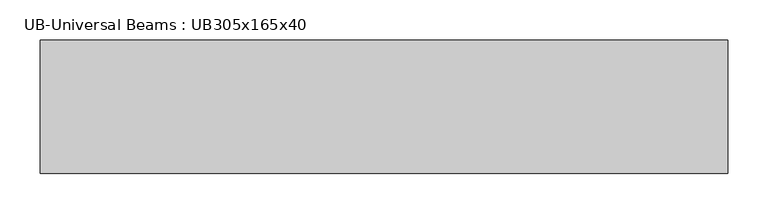
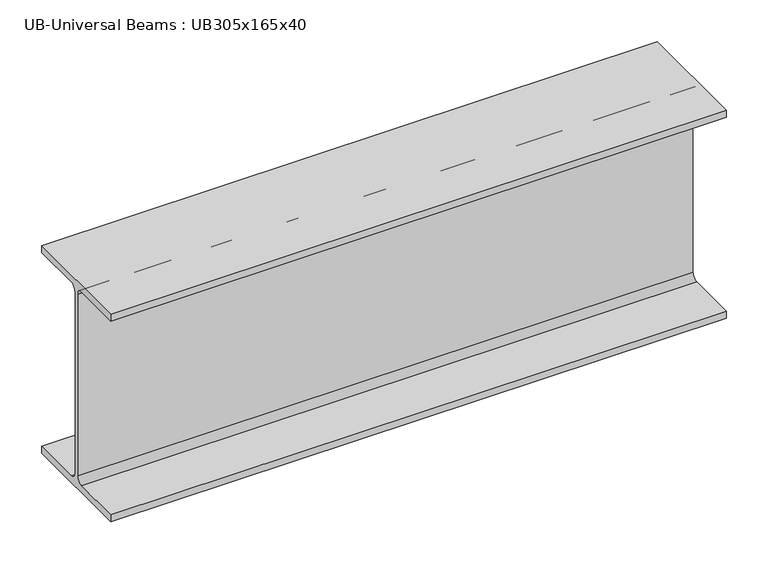
"""IFC4 building model written with IfcOpenShell, lengths in millimetres: beam geometry, UB-Universal Beams : UB305x165x40."""

from ifc_helpers import new_model, si_unit, point, frame, frame_2d, origin, place, context, project, spatial, polyline, circle_curve, trimmed, segment, composite_curve, outline, extrude, source, transform, mapped, element, save


def ub_universal_beams_ub305x165x40_4bff7ce7(model_context):
    return source(origin(), model_context, "Body", "SweptSolid", [
        extrude(outline(composite_curve([segment(polyline([(82.5, -141.5), (82.5, -151.7), (-82.5, -151.7), (-82.5, -141.5), (-11.9, -141.5)]), True, "CONTINUOUS"), segment(trimmed(circle_curve(frame_2d((-11.9, -132.6)), 8.9), [point((-11.9, -141.5))], [point((-3.0, -132.6))], True, "CARTESIAN"), True, "CONTINUOUS"), segment(polyline([(-3.0, -132.6), (-3.0, 132.6)]), True, "CONTINUOUS"), segment(trimmed(circle_curve(frame_2d((-11.9, 132.6)), 8.9), [point((-3.0, 132.6))], [point((-11.9, 141.5))], True, "CARTESIAN"), True, "CONTINUOUS"), segment(polyline([(-11.9, 141.5), (-82.5, 141.5), (-82.5, 151.7), (82.5, 151.7), (82.5, 141.5), (11.9, 141.5)]), True, "CONTINUOUS"), segment(trimmed(circle_curve(frame_2d((11.9, 132.6)), 8.9), [point((11.9, 141.5))], [point((3.0, 132.6))], True, "CARTESIAN"), True, "CONTINUOUS"), segment(polyline([(3.0, 132.6), (3.0, -132.6)]), True, "CONTINUOUS"), segment(trimmed(circle_curve(frame_2d((11.9, -132.6)), 8.9), [point((3.0, -132.6))], [point((11.9, -141.5))], True, "CARTESIAN"), True, "CONTINUOUS"), segment(polyline([(11.9, -141.5), (82.5, -141.5)]), True, "CONTINUOUS")], self_intersect=False)), frame((-435.6, 0.0, 0.0), z_axis=(1.0, 0.0, 0.0), x_axis=(0.0, 1.0, 0.0)), (0.0, 0.0, 1.0), 849.9),
    ])


if __name__ == "__main__":
    model = new_model("IFC4")
    model_context = context("Model", 3, world=origin())
    ifc_project = project(units=[si_unit("LENGTHUNIT", "METRE", prefix="MILLI")], contexts=[model_context])
    site = spatial("IfcSite", under=ifc_project)
    building = spatial("IfcBuilding", under=site)
    placement = place(None, origin())
    ub_universal_beams_ub305x165x40_shape = ub_universal_beams_ub305x165x40_4bff7ce7(model_context)
    element("IfcBeam", 1, ObjectType="UB-Universal Beams : UB305x165x40", at=placement, inside=building, context=model_context, shape_type="MappedRepresentation", body=[
        mapped(ub_universal_beams_ub305x165x40_shape, transform((0.0, 0.0, 0.0), x_axis=(1.0, 0.0, 0.0), y_axis=(0.0, 1.0, 0.0), z_axis=(0.0, 0.0, 1.0))),
    ])
    save(model, "model.ifc")

# Revit data of these elements
# Type "UB-Universal Beams : UB305x165x40"
#   Section Name Key = "UB305X165X40"
#   Width = 16.5 cm
#   Web Thickness = 0.6 cm
#   Web Fillet = 0.89 cm
#   Warping Constant = 164000.0 cm⁶
#   Torsional Moment of Inertia = 14.70 cm⁴
#   Section Area = 51.3 cm²
#   Plastic Modulus weak axis = 142.0 cm³
#   Plastic Modulus strong axis = 623.0 cm³
#   Nominal Weight = 40.2999 kgf/m
#   Moment of Inertia weak axis = 764.00 cm⁴
#   Moment of Inertia strong axis = 8503.00 cm⁴
#   Height = 30.34 cm
#   Flange Thickness = 1.02 cm
#   Elastic Modulus weak axis = 92.6 cm³
#   Elastic Modulus strong axis = 560.0 cm³
#   Centroid Vertical = 15.17 cm
#   Centroid Horizontal = 8.25 cm
#   Bolt Spacing = 9.0 cm
#   Length [instance default] = 1500 mm
#   Structural Material [instance default] = Metal - Steel 43-275
#   Type Comments = ""
#   Assembly Code = ""
# Element 1 (IfcBeam, "UB-Universal Beams : UB305x165x40")
#   Materials on its faces: "Metal - Steel 43-275"
# Materials
#   "Metal - Steel 43-275": class "Metal", colour RGB 247 247 247, transparency 0, Cost = 0
